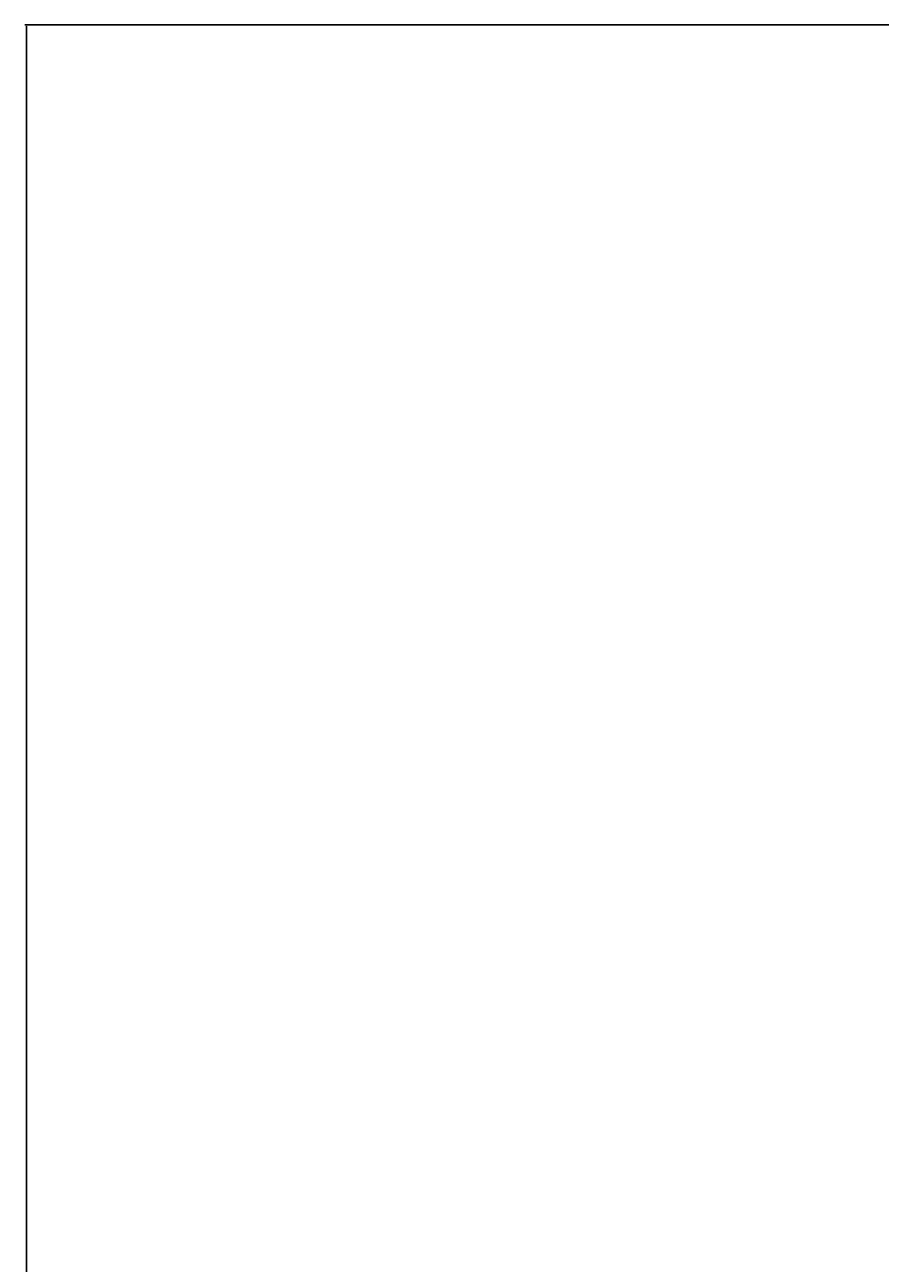
# Model space of a CAD drawing. Units: inches. Extents: x 3731 to 4318, y 1310 to 2388.
# Tile 34 of 57: x 3731 to 3833, y 2192 to 2338. Entities that reach past the tile are written whole.
import ezdxf

# ---------------------------------------------------------------- set-up
doc = ezdxf.new("R2010")
doc.units = ezdxf.units.IN
doc.layers.add('A-ANNO-DIMS', color=2, linetype='Continuous', lineweight=18)
doc.styles.get("Standard").update_dxf_attribs({"font": 'arial.ttf'})
doc.dimstyles.get("Standard").update_dxf_attribs({"dimtxt": 0.18, "dimasz": 0.18, "dimexe": 0.18, "dimexo": 0.0625, "dimgap": 0.09, "dimtad": 0, "dimtih": 1, "dimtoh": 1, "dimdec": 4, "dimzin": 0, "dimdsep": 46, "dimtxsty": 'Standard', "dimcen": 0.09, "dimadec": 0, "dimazin": 0, "dimtfac": 1, "dimtdec": 4, "dimtofl": 0, "dimtmove": 0, "dimatfit": 3, "dimfxl": 1, "dimtolj": 1, "dimtzin": 0, "dimarcsym": 0})

# ---------------------------------------------------------------- blocks, each defined once
blk = doc.blocks.new('*D33')
at = {"layer": 'A-ANNO-DIMS', "color": 0, "lineweight": -2, "transparency": 16777216}
for p, q in [((3835.15, 2338.38), (3731.41, 2338.38)), ((3731.59, 2338.2), (3731.59, 1849.06)), ((3731.59, 1359.56), (3731.59, 1848.7)), ((3835.15, 1359.38), (3731.41, 1359.38))]:
    blk.add_line(p, q, dxfattribs=at)
at = {"layer": 'A-ANNO-DIMS', "color": 0, "transparency": 16777216}
for points in [[(3731.56, 2338.2), (3731.62, 2338.2), (3731.59, 2338.38)], [(3731.56, 1359.56), (3731.62, 1359.56), (3731.59, 1359.38)]]:
    blk.add_solid(points, dxfattribs=at)
at = {"layer": 'Defpoints', "color": 0, "transparency": 16777216}
for p in [(3731.59, 2338.38), (3835.21, 2338.38), (3835.21, 1359.38)]:
    blk.add_point(p, dxfattribs=at)
at = {"layer": 'A-ANNO-DIMS', "color": 0, "transparency": 16777216, "insert": (3731.59, 1848.88), "char_height": 0.18, "attachment_point": 5}
blk.add_mtext('\\A1;979', dxfattribs=at)

msp = doc.modelspace()

# ---------------------------------------------------------------- dimensions: what is measured, and where the dimension line sits
at = {"layer": 'A-ANNO-DIMS'}
dim = msp.add_linear_dim(base=(3731.59, 2338.38), p1=(3835.21, 1359.38), p2=(3835.21, 2338.38), angle=90, dimstyle='Standard', override={"dimdec": 0, "dimlfac": 1, "dimrnd": 0, "dimzin": 0, "dimdsep": 46, "dimlunit": 2}, dxfattribs=at)
dim.commit()
dim.dimension.update_dxf_attribs({"geometry": '*D33', "text_midpoint": (3731.59, 1848.88)})

doc.saveas('drawing.dxf')
